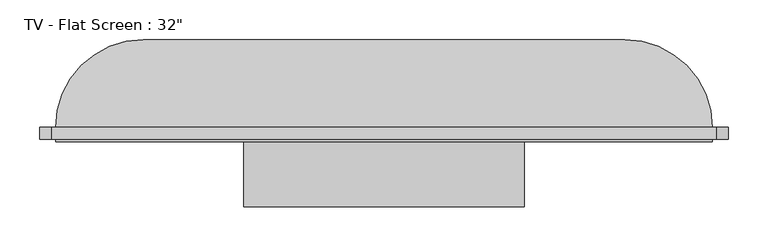
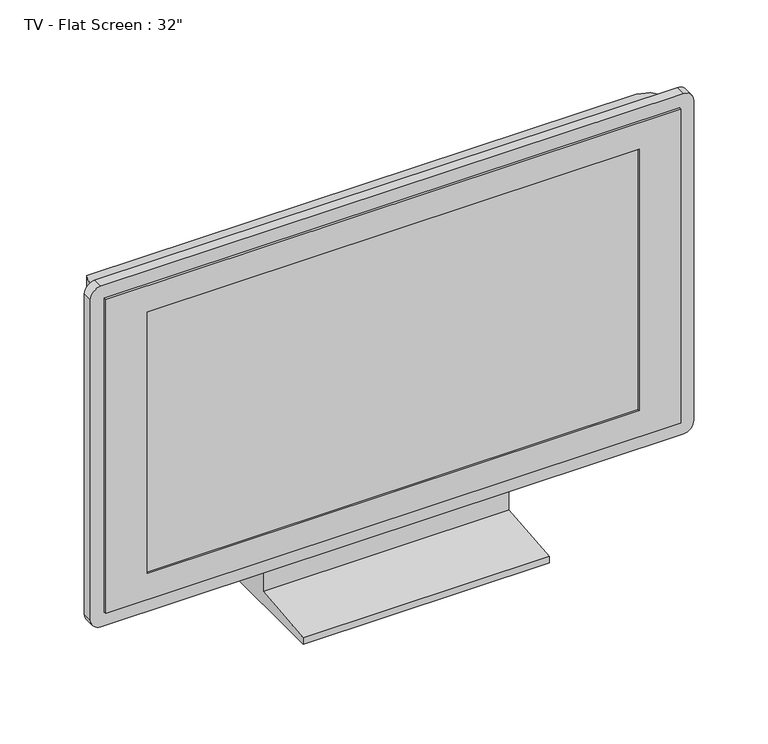
"""IFC4 building model written with IfcOpenShell, lengths in millimetres: furniture geometry."""

from ifc_helpers import new_model, si_unit, point, frame, frame_2d, origin, place, context, project, spatial, polyline, circle_curve, ellipse_curve, trimmed, segment, composite_curve, outline, extrude, faceted_brep, source, transform, mapped, element, save
from ifc_brep_helpers import plane_surface, cylinder_surface, advanced_brep


def furniture_56245f3a(model_context):
    return source(origin(), model_context, "Body", "SolidModel", [
        extrude(outline(polyline([(-51.4613764, 80.0), (-1.4613764, 80.0), (48.5386236, 0.0), (-151.4613764, 0.0), (-151.4613764, 10.0), (-51.4613764, 20.0), (-51.4613764, 80.0)])), frame((-180.4346678, 0.0, 0.0), z_axis=(1.0, 0.0, 0.0), x_axis=(0.0, 1.0, 0.0)), (0.0, 0.0, 1.0), 352.9803073),
        faceted_brep([(409.0357931, -69.4613764, 557.1392838), (-416.9248214, -69.4613764, 557.1392838), (-416.9248214, -69.4613764, 80.0), (409.0357931, -69.4613764, 80.0), (-356.9248214, -69.4613764, 517.1392838), (349.0357931, -69.4613764, 517.1392838), (349.0357931, -69.4613764, 120.0), (-356.9248214, -69.4613764, 120.0), (409.0357931, -51.4613764, 557.1392838), (409.0357931, -51.4613764, 80.0), (-416.9248214, -51.4613764, 80.0), (-416.9248214, -51.4613764, 557.1392838), (-356.9248214, -66.4613764, 517.1392838), (-356.9248214, -66.4613764, 120.0), (349.0357931, -66.4613764, 120.0), (349.0357931, -66.4613764, 517.1392838)], [[[0, 1, 2, 3], [4, 5, 6, 7]], [[8, 9, 10, 11]], [[1, 0, 8, 11]], [[2, 1, 11, 10]], [[3, 2, 10, 9]], [[0, 3, 9, 8]], [[12, 13, 14, 15]], [[12, 15, 5, 4]], [[15, 14, 6, 5]], [[14, 13, 7, 6]], [[13, 12, 4, 7]]]),
        extrude(outline(composite_curve([segment(polyline([(577.1392838, 414.0357931), (577.1392838, -421.9248214)]), True, "CONTINUOUS"), segment(trimmed(circle_curve(frame_2d((562.1392838, -421.9248214)), 15.0), [point((577.1392838, -421.9248214))], [point((562.1392838, -436.9248214))], False, "CARTESIAN"), True, "CONTINUOUS"), segment(polyline([(562.1392838, -436.9248214), (75.0, -436.9248214)]), True, "CONTINUOUS"), segment(trimmed(circle_curve(frame_2d((75.0, -421.9248214)), 15.0), [point((75.0, -436.9248214))], [point((60.0, -421.9248214))], False, "CARTESIAN"), True, "CONTINUOUS"), segment(polyline([(60.0, -421.9248214), (60.0, 414.0357931)]), True, "CONTINUOUS"), segment(trimmed(circle_curve(frame_2d((75.0, 414.0357931)), 15.0), [point((60.0, 414.0357931))], [point((75.0, 429.0357931))], False, "CARTESIAN"), True, "CONTINUOUS"), segment(polyline([(75.0, 429.0357931), (562.1392838, 429.0357931)]), True, "CONTINUOUS"), segment(trimmed(circle_curve(frame_2d((562.1392838, 414.0357931)), 15.0), [point((562.1392838, 429.0357931))], [point((577.1392838, 414.0357931))], False, "CARTESIAN"), True, "CONTINUOUS")], self_intersect=False), holes=[polyline([(557.1392838, 409.0357931), (80.0, 409.0357931), (80.0, -416.9248214), (557.1392838, -416.9248214), (557.1392838, 409.0357931)])]), frame((0.0, -66.4613764, 0.0), z_axis=(0.0, 1.0, 0.0), x_axis=(0.0, 0.0, 1.0)), (0.0, 0.0, 1.0), 15.0),
        advanced_brep(
        [(-416.9248214, -51.4613764, 80.0), (409.0357931, -51.4613764, 80.0), (409.0357931, -51.4613764, 557.1392838), (-416.9248214, -51.4613764, 557.1392838), (299.0357931, 58.5386236, 80.0), (-306.9248214, 58.5386236, 80.0), (-306.9248214, 58.5386236, 447.1392838), (299.0357931, 58.5386236, 447.1392838)],
        [
            (0, 1),
            (1, 2),
            (2, 3),
            (3, 0),
            (4, 5),
            (5, 6),
            (6, 7),
            (7, 4),
            (0, 5, circle_curve(frame((-306.9248214, -51.4613764, 80.0), z_axis=(0.0, 0.0, -1.0), x_axis=(-1.0, 0.0, 0.0)), 110.0)),
            (4, 1, circle_curve(frame((299.0357931, -51.4613764, 80.0), z_axis=(0.0, 0.0, -1.0), x_axis=(1.0, 0.0, 0.0)), 110.0)),
            (7, 2, ellipse_curve(frame((299.0357931, -51.4613764, 447.1392838), z_axis=(0.7071067811865475, 0.0, -0.7071067811865475), x_axis=(0.7071067811865474, 0.0, 0.7071067811865476)), 155.5634919, 110.0)),
            (6, 3, ellipse_curve(frame((-306.9248214, -51.4613764, 447.1392838), z_axis=(0.7071067811865475, 0.0, 0.7071067811865475), x_axis=(-0.7071067811865476, 0.0, 0.7071067811865474)), 155.5634919, 110.0)),
        ],
        [
            plane_surface(frame((-416.9248214, -51.4613764, 557.1392838), z_axis=(0.0, -1.0, 0.0), x_axis=(-1.0, 0.0, 0.0))),
            plane_surface(frame((-416.9248214, 58.5386236, 557.1392838), z_axis=(0.0, 1.0, 0.0), x_axis=(1.0, 0.0, 0.0))),
            plane_surface(frame((-416.9248214, -51.4613764, 80.0), z_axis=(0.0, 0.0, -1.0), x_axis=(0.0, 1.0, 0.0))),
            cylinder_surface(frame((299.0357931, -51.4613764, 80.0), z_axis=(0.0, 0.0, 1.0), x_axis=(1.0, 0.0, 0.0)), 110.0),
            cylinder_surface(frame((409.0357931, -51.4613764, 447.1392838), z_axis=(-1.0, 0.0, 0.0), x_axis=(0.0, 0.0, 1.0)), 110.0),
            cylinder_surface(frame((-306.9248214, -51.4613764, 557.1392838), z_axis=(0.0, 0.0, -1.0), x_axis=(-1.0, 0.0, 0.0)), 110.0),
        ],
        [
            (0, [[1, 2, 3, 4]]),
            (1, [[5, 6, 7, 8]]),
            (2, [[-1, 9, -5, 10]]),
            (3, [[11, -2, -10, -8]]),
            (4, [[-11, -7, 12, -3]]),
            (5, [[-12, -6, -9, -4]]),
        ],
    ),
    ])


if __name__ == "__main__":
    model = new_model("IFC4")
    model_context = context("Model", 3, world=origin())
    ifc_project = project(units=[si_unit("LENGTHUNIT", "METRE", prefix="MILLI")], contexts=[model_context])
    site = spatial("IfcSite", under=ifc_project)
    building = spatial("IfcBuilding", under=site)
    placement = place(None, origin())
    furniture_shape = furniture_56245f3a(model_context)
    element("IfcFurniture", 1, ObjectType="TV - Flat Screen : 32\"", at=placement, inside=building, context=model_context, shape_type="MappedRepresentation", body=[
        mapped(furniture_shape, transform((0.0, 0.0, 0.0), x_axis=(1.0, 0.0, 0.0), y_axis=(0.0, 1.0, 0.0), z_axis=(0.0, 0.0, 1.0))),
    ])
    save(model, "model.ifc")

# Revit data of these elements
# Type "TV - Flat Screen : 32\""
#   SinAng = 0' - 0.0193"
#   L = 2' - 3.79372"
#   H = 1' - 3.6354"
#   Thickness = 0' - 4.33071"
#   Diagonal = 2' - 7.88976"
#   CosAng = 0' - 0.03431"
#   Stand [instance default] = yes
#   Default Elevation = 0
# Element 1 (IfcFurniture, "TV - Flat Screen : 32\"")
#   Materials on its faces: "TV - Black", "TV - Glass", "TV - Screen"
# Materials
#   "TV - Black": colour RGB 49 49 49, transparency 0
#   "TV - Glass": colour RGB 157 157 157, transparency 0.9
#   "TV - Screen": colour RGB 0 0 0, transparency 0
